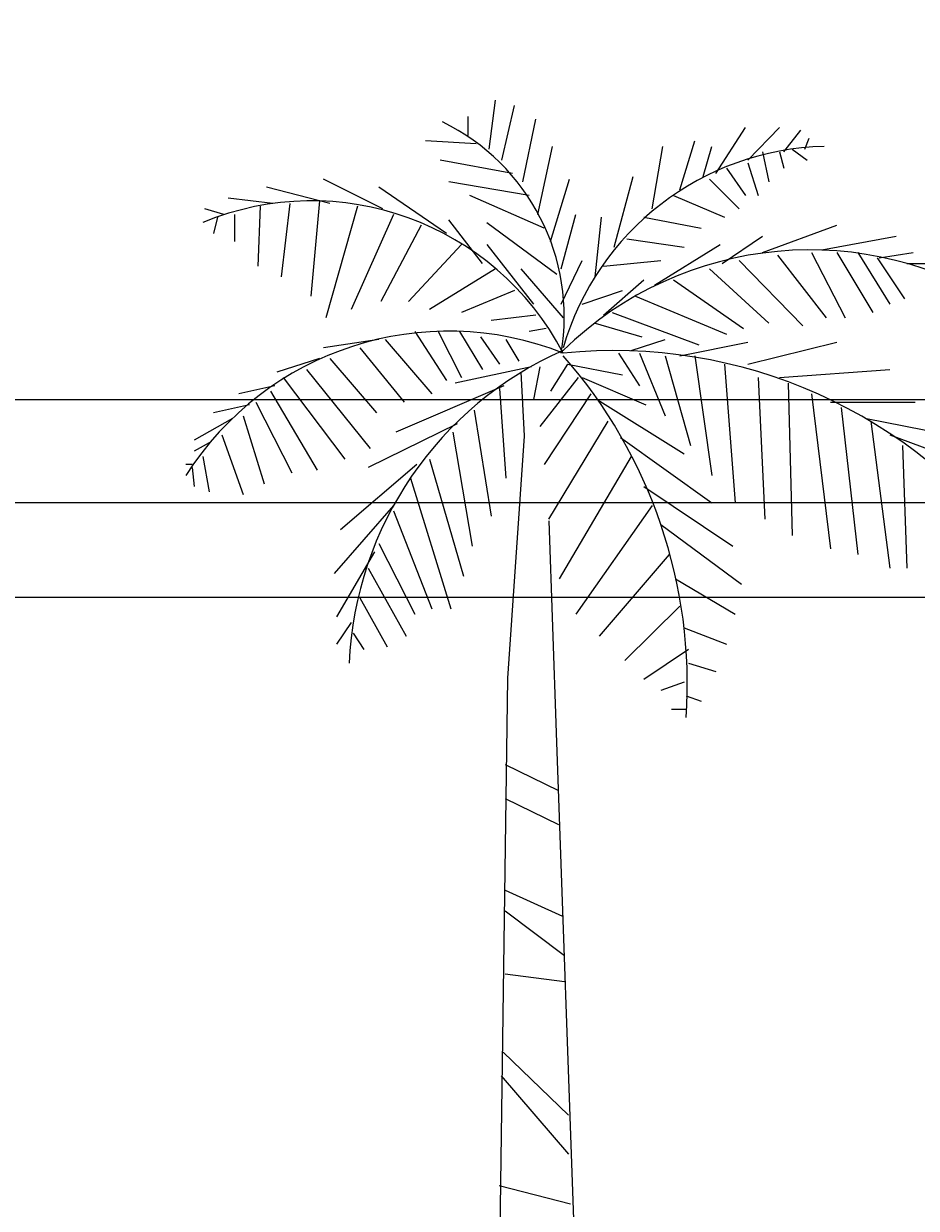
# Model space of a CAD drawing. Units: inches. Extents: x -13 to 809, y 112 to 656.
# Tile 48 of 55: x 621 to 702, y 251 to 359. Entities that reach past the tile are written whole.
import ezdxf

# ---------------------------------------------------------------- set-up
doc = ezdxf.new("R2010")
doc.units = ezdxf.units.IN
doc.header["$MEASUREMENT"] = 0
doc.layers.add('A-ANNO-DIMS', color=2, linetype='Continuous', lineweight=18)
doc.layers.add('L-PLNT', color=3, linetype='Continuous', lineweight=18)
doc.styles.get("Standard").update_dxf_attribs({"font": 'arial.ttf'})
doc.dimstyles.get("Standard").update_dxf_attribs({"dimtxt": 0.625, "dimasz": 0.18, "dimexe": 0.18, "dimexo": 0.0625, "dimgap": 0.09, "dimtad": 0, "dimtih": 1, "dimtoh": 1, "dimdec": 4, "dimzin": 0, "dimdsep": 46, "dimlunit": 4, "dimtxsty": 'Standard', "dimcen": 0.09, "dimadec": 0, "dimazin": 0, "dimtfac": 1, "dimtdec": 4, "dimtofl": 0, "dimtmove": 0, "dimatfit": 3, "dimfxl": 1, "dimtolj": 1, "dimtzin": 0, "dimarcsym": 0})

# ---------------------------------------------------------------- blocks, each defined once
blk = doc.blocks.new('Tree - palm elevation')
for p, q in [((-5.567, 196.707), (-4.987, 201.167)), ((-7.5, 199.68), (-7.5, 197.946)), ((-4.407, 195.716), (-3.247, 200.672)), ((-2.474, 193.733), (-1.315, 199.433)), ((15.116, 194.477), (17.822, 198.689)), ((18.015, 195.716), (20.914, 198.689)), ((21.301, 196.459), (22.847, 198.441)), ((23.234, 196.707), (23.62, 197.698)), ((-6.727, 197.202), (-11.366, 197.45)), ((-1.121, 190.759), (0.232, 196.955)), ((9.317, 191.255), (10.283, 196.955)), ((11.829, 192.99), (13.182, 197.45)), ((13.956, 194.229), (14.729, 196.955)), ((19.368, 196.459), (19.948, 193.733)), ((20.914, 196.459), (21.301, 194.972)), ((22.074, 196.707), (23.427, 195.716)), ((-3.441, 194.477), (-10.013, 195.716)), ((18.015, 195.468), (18.981, 192.494)), ((16.082, 194.972), (17.822, 192.494)), ((-20.064, 191.751), (-25.863, 193.238)), ((-15.232, 191.255), (-20.644, 193.981)), ((-9.433, 189.025), (-15.618, 193.238)), ((-1.894, 192.494), (-9.24, 193.733)), ((0.038, 188.281), (1.778, 193.981)), ((5.837, 187.786), (7.577, 194.229)), ((14.536, 193.981), (17.242, 191.255)), ((-25.283, 191.751), (-29.342, 192.246)), ((-0.541, 189.52), (-7.307, 192.494)), ((11.25, 192.494), (15.889, 190.512)), ((-29.729, 190.759), (-31.469, 191.255)), ((-26.443, 191.503), (-26.636, 186.051)), ((-23.737, 191.751), (-24.51, 185.06)), ((-21.031, 191.998), (-21.804, 183.325)), ((-17.551, 191.503), (-20.451, 181.343)), ((-30.309, 190.512), (-30.695, 189.025)), ((-28.763, 190.759), (-28.763, 188.281)), ((-14.265, 190.759), (-18.131, 182.086)), ((-6.147, 186.299), (-9.24, 190.264)), ((-5.76, 190.016), (0.618, 185.308)), ((1.005, 185.803), (2.358, 190.759)), ((4.098, 185.06), (4.678, 190.512)), ((8.544, 190.512), (13.763, 189.52)), ((-11.753, 189.768), (-15.425, 182.83)), ((19.368, 187.29), (26.133, 189.768)), ((-8.08, 188.034), (-12.912, 182.83)), ((-5.76, 188.034), (-1.508, 182.582)), ((6.997, 188.529), (12.216, 187.786)), ((9.51, 184.317), (15.502, 188.034)), ((15.695, 186.299), (19.368, 188.777)), ((24.78, 187.538), (31.546, 188.777)), ((20.721, 187.042), (25.167, 181.343)), ((23.814, 187.29), (26.907, 181.343)), ((26.133, 187.29), (29.419, 181.838)), ((28.066, 187.29), (30.966, 182.582)), ((29.806, 186.795), (32.319, 183.078)), ((29.999, 186.795), (33.092, 187.29)), ((-4.987, 185.803), (-10.979, 182.086)), ((-2.668, 185.803), (1.198, 181.343)), ((1.005, 182.582), (2.938, 186.547)), ((4.871, 186.051), (10.09, 186.547)), ((14.536, 185.803), (19.948, 180.847)), ((17.242, 186.547), (23.041, 180.599)), ((32.512, 186.299), (35.218, 186.299)), ((4.871, 181.591), (8.544, 184.812)), ((11.25, 184.812), (17.628, 180.352)), ((-3.247, 183.821), (-8.08, 181.838)), ((2.938, 182.582), (6.61, 183.821)), ((7.77, 183.325), (16.082, 179.856)), ((-1.315, 181.591), (-5.374, 181.095)), ((5.644, 181.838), (13.569, 178.865)), ((-0.348, 180.352), (-1.894, 180.104)), ((4.098, 180.847), (8.35, 179.608)), ((-15.618, 179.36), (-20.644, 178.617)), ((-15.038, 179.36), (-10.786, 174.404)), ((-12.332, 180.104), (-9.433, 175.643)), ((-10.206, 180.104), (-8.08, 175.891)), ((-8.273, 180.104), (-6.147, 176.635)), ((-6.34, 179.608), (-4.6, 177.13)), ((-4.021, 179.36), (-2.861, 177.378)), ((7.384, 178.369), (10.476, 179.36)), ((-17.358, 178.617), (-13.299, 173.661)), ((6.224, 178.121), (8.157, 175.148)), ((8.157, 178.121), (10.476, 172.422)), ((11.829, 177.874), (18.015, 179.113)), ((18.015, 177.13), (26.133, 179.113)), ((-21.031, 177.626), (-24.897, 176.387)), ((-20.064, 177.626), (-15.812, 172.67)), ((1.585, 177.13), (0.038, 174.652)), ((1.585, 177.13), (6.61, 176.139)), ((10.476, 177.874), (12.796, 169.696)), ((13.182, 177.874), (14.729, 166.97)), ((15.889, 177.13), (16.855, 164.492)), ((-22.191, 176.635), (-16.391, 169.448)), ((-1.701, 176.882), (-8.66, 175.396)), ((-2.668, 176.387), (-2.376, 170.594)), ((-0.928, 176.882), (-1.508, 173.909)), ((20.914, 175.891), (30.966, 176.635)), ((-25.09, 175.148), (-28.376, 174.404)), ((-24.317, 175.891), (-18.711, 168.457)), ((-4.214, 175.148), (-14.072, 170.935)), ((-4.6, 174.9), (-4.021, 166.722)), ((2.551, 175.891), (-0.928, 171.431)), ((2.938, 175.891), (8.737, 173.413)), ((18.981, 175.891), (19.561, 163.005)), ((21.688, 175.396), (22.074, 161.518)), ((-25.476, 174.652), (-21.224, 167.466)), ((3.711, 174.404), (-0.541, 167.961)), ((4.291, 173.909), (12.216, 168.953)), ((23.814, 174.404), (25.554, 160.279)), ((-27.409, 173.413), (-30.695, 172.67)), ((-26.829, 173.661), (-23.544, 167.218)), ((-6.92, 172.917), (-5.374, 163.253)), ((25.554, 173.661), (33.285, 173.661)), ((26.52, 173.165), (28.066, 159.784)), ((-28.956, 172.174), (-32.435, 170.192)), ((-27.989, 172.422), (-26.056, 166.227)), ((-8.466, 171.678), (-16.585, 167.713)), ((5.257, 171.926), (-0.155, 163.005)), ((28.839, 172.174), (36.378, 170.687)), ((29.226, 171.926), (30.966, 158.545)), ((-29.922, 170.687), (-27.989, 165.235)), ((-8.853, 170.935), (-7.113, 160.527)), ((30.966, 170.687), (38.891, 167.713)), ((-31.082, 169.944), (-32.435, 169.2)), ((6.417, 170.439), (14.729, 164.492)), ((32.126, 169.696), (32.512, 158.545)), ((-31.662, 168.705), (-31.082, 165.483)), ((-10.979, 168.457), (-7.887, 157.801)), ((7.384, 168.705), (0.812, 157.553)), ((-32.628, 167.961), (-33.208, 167.961)), ((-32.628, 167.713), (-32.435, 165.979)), ((-12.139, 167.961), (-19.098, 162.014)), ((-12.719, 166.722), (-9.046, 154.828)), ((8.544, 165.979), (16.662, 160.527)), ((-14.265, 164.244), (-19.678, 158.049)), ((9.317, 164.244), (2.358, 154.332)), ((-14.265, 163.749), (-10.786, 154.828)), ((10.09, 162.51), (17.435, 157.058)), ((-16.005, 160.031), (-19.484, 154.084)), ((-15.618, 160.775), (-12.332, 154.332)), ((10.863, 159.784), (4.484, 152.35)), ((-16.585, 158.545), (-13.106, 152.35)), ((11.443, 157.553), (16.855, 154.332)), ((-17.358, 155.819), (-14.845, 151.358)), ((11.829, 155.075), (6.804, 150.119)), ((-18.131, 153.589), (-19.484, 151.606)), ((-17.938, 152.597), (-16.972, 151.111)), ((12.216, 153.093), (16.082, 151.606)), ((12.603, 151.111), (8.544, 148.385)), ((12.603, 149.872), (15.116, 149.128)), ((12.216, 148.137), (10.09, 147.393)), ((12.409, 146.898), (13.763, 146.402)), ((12.409, 145.659), (11.056, 145.659)), ((-4.081, 140.645), (0.753, 138.261)), ((-4.081, 137.547), (0.753, 135.163)), ((-4.081, 129.205), (1.124, 126.821)), ((-4.081, 127.298), (1.31, 123.246)), ((-4.081, 121.578), (1.31, 120.863)), ((-4.267, 114.428), (1.682, 108.708)), ((-4.453, 112.283), (1.682, 105.133)), ((-4.639, 102.273), (1.868, 100.604))]:
    blk.add_line(p, q)
for points in [[(-2.363, 170.553), (-3.88, 148.505), (-4.988, 69.634), (-3.325, 24.869), (0, 0)], [(-0.116, 162.848), (0.554, 143.532), (2.217, 96.635), (3.88, 44.054), (7.76, 12.079), (11.64, 0)]]:
    blk.add_lwpolyline(points)
for centre, radius, start, end in [((-18.427, 181.448), 19.715, 350.285, 64.11229), ((25.595, 171.567), 25.395, 91.40319, 163.882), ((-21.738, 166.094), 25.899, 27.67115, 112.5305), ((23.687, 155.341), 32.188, 56.19272, 134.3213), ((-9.259, 151.732), 28.386, 68.38311, 147.5322), ((14.394, 148.393), 32.752, 113.7592, 177.4133), ((5.828, 132.718), 45.639, 35.98777, 95.82273), ((-32.8, 147.923), 45.309, 356.1943, 41.37848)]:
    blk.add_arc(centre, radius, start, end)
blk = doc.blocks.new('*D31')
at = {"layer": 'A-ANNO-DIMS', "color": 0, "lineweight": -2, "transparency": 16777216}
for p, q in [((621.07, 617.78), (807.77, 617.78)), ((807.59, 617.6), (807.59, 384.56)), ((807.59, 150.7), (807.59, 383.74)), ((621.07, 150.52), (807.77, 150.52))]:
    blk.add_line(p, q, dxfattribs=at)
at = {"layer": 'A-ANNO-DIMS', "color": 0, "transparency": 16777216}
for points in [[(807.56, 617.6), (807.62, 617.6), (807.59, 617.78)], [(807.56, 150.7), (807.62, 150.7), (807.59, 150.52)]]:
    blk.add_solid(points, dxfattribs=at)
at = {"layer": 'Defpoints', "color": 0, "transparency": 16777216}
for p in [(621.01, 617.78), (807.59, 617.78), (621.01, 150.52)]:
    blk.add_point(p, dxfattribs=at)
at = {"layer": 'A-ANNO-DIMS', "color": 0, "transparency": 16777216, "insert": (807.59, 384.15), "char_height": 0.625, "attachment_point": 5}
blk.add_mtext('\\A1;467.3', dxfattribs=at)
blk = doc.blocks.new('*D46')
at = {"layer": 'A-ANNO-DIMS', "color": 0, "lineweight": -2, "transparency": 16777216}
for p, q in [((160.98, 408.79), (807.77, 408.79)), ((807.59, 408.61), (807.59, 367.07)), ((807.59, 324.7), (807.59, 366.25)), ((160.98, 324.52), (807.77, 324.52))]:
    blk.add_line(p, q, dxfattribs=at)
at = {"layer": 'A-ANNO-DIMS', "color": 0, "transparency": 16777216}
for points in [[(807.56, 408.61), (807.62, 408.61), (807.59, 408.79)], [(807.56, 324.7), (807.62, 324.7), (807.59, 324.52)]]:
    blk.add_solid(points, dxfattribs=at)
at = {"layer": 'Defpoints', "color": 0, "transparency": 16777216}
for p in [(160.92, 408.79), (807.59, 408.79), (160.92, 324.52)]:
    blk.add_point(p, dxfattribs=at)
at = {"layer": 'A-ANNO-DIMS', "color": 0, "transparency": 16777216, "insert": (807.59, 366.66), "char_height": 0.625, "attachment_point": 5}
blk.add_mtext('\\A1;84.27', dxfattribs=at)
blk = doc.blocks.new('*D48')
at = {"layer": 'A-ANNO-DIMS', "color": 0, "lineweight": -2, "transparency": 16777216}
for p, q in [((319.57, 444.52), (807.77, 444.52)), ((807.59, 444.34), (807.59, 384.93)), ((807.59, 324.7), (807.59, 384.11)), ((319.57, 324.52), (807.77, 324.52))]:
    blk.add_line(p, q, dxfattribs=at)
at = {"layer": 'A-ANNO-DIMS', "color": 0, "transparency": 16777216}
for points in [[(807.56, 444.34), (807.62, 444.34), (807.59, 444.52)], [(807.56, 324.7), (807.62, 324.7), (807.59, 324.52)]]:
    blk.add_solid(points, dxfattribs=at)
at = {"layer": 'Defpoints', "color": 0, "transparency": 16777216}
for p in [(319.51, 444.52), (807.59, 444.52), (319.51, 324.52)]:
    blk.add_point(p, dxfattribs=at)
at = {"layer": 'A-ANNO-DIMS', "color": 0, "transparency": 16777216, "insert": (807.59, 384.52), "char_height": 0.625, "attachment_point": 5}
blk.add_mtext('\\A1;120', dxfattribs=at)
blk = doc.blocks.new('*D106')
at = {"layer": 'A-ANNO-DIMS', "color": 0, "lineweight": -2, "transparency": 16777216}
for p, q in [((319.57, 315.14), (807.77, 315.14)), ((807.59, 314.96), (807.59, 311.24)), ((807.59, 306.7), (807.59, 310.42)), ((337.57, 306.52), (807.77, 306.52))]:
    blk.add_line(p, q, dxfattribs=at)
at = {"layer": 'A-ANNO-DIMS', "color": 0, "transparency": 16777216}
for points in [[(807.56, 314.96), (807.62, 314.96), (807.59, 315.14)], [(807.56, 306.7), (807.62, 306.7), (807.59, 306.52)]]:
    blk.add_solid(points, dxfattribs=at)
at = {"layer": 'Defpoints', "color": 0, "transparency": 16777216}
for p in [(319.51, 315.14), (807.59, 315.14), (337.51, 306.52)]:
    blk.add_point(p, dxfattribs=at)
at = {"layer": 'A-ANNO-DIMS', "color": 0, "transparency": 16777216, "insert": (807.59, 310.83), "char_height": 0.625, "attachment_point": 5}
blk.add_mtext('\\A1;8.624', dxfattribs=at)

msp = doc.modelspace()

# ---------------------------------------------------------------- block references
at = {"layer": 'L-PLNT'}
msp.add_blockref('Tree - palm elevation', (668.9925, 150.6343), dxfattribs=at)

# ---------------------------------------------------------------- dimensions: what is measured, and where the dimension line sits
at = {"layer": 'A-ANNO-DIMS'}
for base, p1, p2, override, picture, middle in [((807.5888, 617.7828), (621.008, 150.5199), (621.008, 617.7828), {"dimdec": 1, "dimlfac": 1, "dimrnd": 0, "dimzin": 0, "dimdsep": 46, "dimlunit": 2}, '*D31', (807.5888, 384.1514)), ((807.5888, 444.5199), (319.5074, 324.5199), (319.5074, 444.5199), {"dimdec": 0, "dimlfac": 1, "dimrnd": 0, "dimzin": 0, "dimdsep": 46, "dimlunit": 2}, '*D48', (807.5888, 384.5199)), ((807.5888, 408.7939), (160.9184, 324.5199), (160.9184, 408.7939), {"dimdec": 2, "dimlfac": 1, "dimrnd": 0, "dimzin": 0, "dimdsep": 46, "dimlunit": 2}, '*D46', (807.5888, 366.6569)), ((807.5888, 315.1435), (337.5074, 306.5199), (319.5074, 315.1435), {"dimdec": 3, "dimlfac": 1, "dimrnd": 0, "dimzin": 0, "dimdsep": 46, "dimlunit": 2}, '*D106', (807.5888, 310.8317))]:
    dim = msp.add_linear_dim(base=base, p1=p1, p2=p2, angle=90, dimstyle='Standard', override=override, dxfattribs=at)
    dim.commit()
    dim.dimension.update_dxf_attribs({"geometry": picture, "text_midpoint": middle})

doc.saveas('drawing.dxf')
